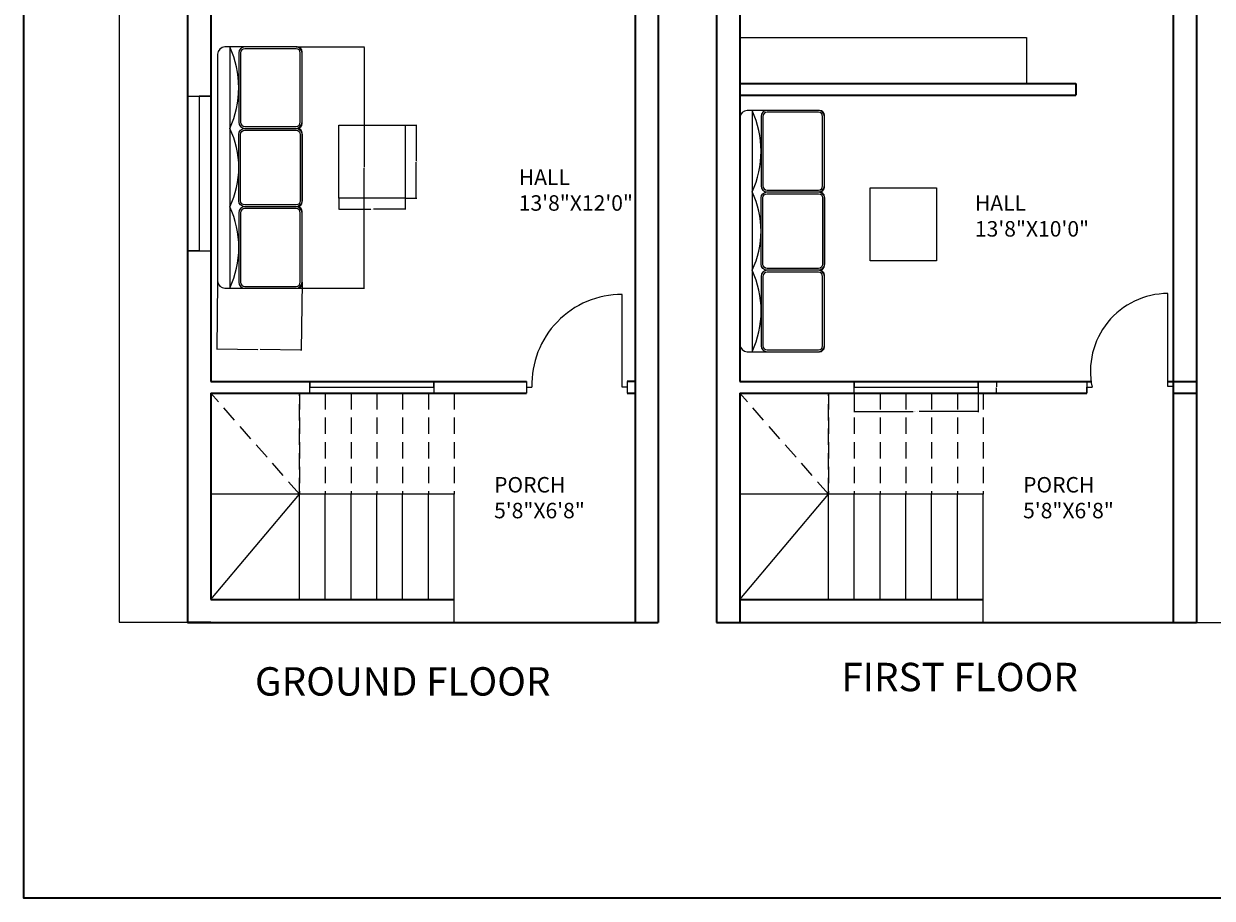
# Model space of a CAD drawing. Units: inches. Extents: x 2169 to 3181, y 1824 to 2912.
# Tile 1 of 5: x 2169 to 2630, y 1824 to 2163. Entities that reach past the tile are written whole.
import ezdxf

# ---------------------------------------------------------------- set-up
doc = ezdxf.new("R2010")
doc.units = ezdxf.units.IN
doc.linetypes.add('DASHED2', pattern=[9.525, 6.35, -3.175])
for name, color, linetype, lineweight in [('A-ANNO-DIMS', 2, 'Continuous', 18), ('A-ANNO-TITL', 7, 'Continuous', 25), ('A-ANNO-TTLB', 7, 'Continuous', 35), ('A-AREA-IDEN', 7, 'Continuous', 18), ('A-DOOR', 3, 'Continuous', 18), ('A-FLOR-CASE', 8, 'Continuous', 18), ('A-FLOR-STRS', 7, 'Continuous', 18), ('A-FLOR-STRS-OVHD', 253, 'DASHED2', 13), ('A-FURN', 8, 'Continuous', 18), ('A-GLAZ', 4, 'Continuous', 18), ('A-WALL', 7, 'Continuous', 35)]:
    doc.layers.add(name, color=color, linetype=linetype, lineweight=lineweight)
doc.styles.get("Standard").update_dxf_attribs({"font": 'arial.ttf'})
doc.dimstyles.get("Standard").update_dxf_attribs({"dimtxt": 0.18, "dimasz": 0.18, "dimexe": 0.18, "dimexo": 0.0625, "dimgap": 0.09, "dimtad": 0, "dimtih": 1, "dimtoh": 1, "dimdec": 4, "dimzin": 0, "dimdsep": 46, "dimtxsty": 'Standard', "dimcen": 0.09, "dimadec": 0, "dimazin": 0, "dimtfac": 1, "dimtdec": 4, "dimtofl": 0, "dimtmove": 0, "dimatfit": 3, "dimfxl": 1, "dimtolj": 1, "dimtzin": 0, "dimarcsym": 0})

# ---------------------------------------------------------------- blocks, each defined once
blk = doc.blocks.new('DOOR-ENTRY-G-36IN')
for p, q in [((0, 0), (0, 36)), ((-37.01, 2.25), (-37.01, -2.25)), ((2, 2.25), (2, -2.25)), ((-37.01, 0), (-35.01, 0)), ((2, 0), (0, 0))]:
    blk.add_line(p, q)
blk.add_arc((0, 0.98), 35.02, 90, 181.6016)
blk = doc.blocks.new('DOOR-ENTRY-U-36IN')
for p, q in [((0, 0), (0, 36)), ((-31.41, 1.93), (-31.41, 1.93)), ((-31.41, 1.93), (-31.41, -2.57)), ((2, 0), (0, 0)), ((-31.41, -2.57), (-31.41, -0.32)), ((-31.41, -0.32), (-31.41, -0.32)), ((-31.41, -0.32), (-29.41, -0.32))]:
    blk.add_line(p, q)
blk.add_arc((0, 5.93), 30.07, 90, 192.0072)
blk = doc.blocks.new('WIN-60IN')
for p, q in [((4.5, 60), (0, 60)), ((0, 60), (9, 60)), ((4.5, 0), (4.5, 60)), ((0, 0), (9, 0)), ((9, 0), (4.5, 0)), ((9, 0), (9, 0))]:
    blk.add_line(p, q)
blk = doc.blocks.new('WIN-48IN')
for p, q in [((0, 0), (0, 4.5)), ((0, 4.5), (0, 2.25)), ((0, 2.25), (48, 2.25)), ((48, 2.25), (48, 4.5)), ((48, 4.5), (48, 0))]:
    blk.add_line(p, q)
blk = doc.blocks.new('STAIR-RETURN-LOWER')
for p, q in [((94.36, 49.81), (0, 49.81)), ((0, 9), (34.36, 49.81)), ((34.36, 9), (34.36, 49.81)), ((44.36, 9), (44.36, 49.81)), ((54.36, 9), (54.36, 49.81)), ((64.36, 9), (64.36, 49.81)), ((74.36, 9), (74.36, 49.81)), ((84.36, 9), (84.36, 49.81)), ((94.36, 0), (94.36, 49.81))]:
    blk.add_line(p, q)
blk = doc.blocks.new('STAIR-RETURN-UPPER')
for p, q in [((34.36, 0), (0, 39.19)), ((34.36, 0), (34.36, 39.19)), ((34.36, 39.19), (34.36, 0)), ((44.36, 39.19), (44.36, 0)), ((54.36, 39.19), (54.36, 0)), ((64.36, 39.19), (64.36, 0)), ((74.36, 39.19), (74.36, 0)), ((84.36, 39.19), (84.36, 0)), ((94.36, 39.19), (94.36, 0))]:
    blk.add_line(p, q)
blk = doc.blocks.new('TABLE-COFFEE')
blk.add_lwpolyline([(0, 28.27), (25.7, 28.27), (25.7, 0), (0, 0)], close=True)
blk = doc.blocks.new('*D21')
at = {"layer": 'A-ANNO-DIMS', "color": 0, "lineweight": -2, "transparency": 16777216}
for p, q in [((2490.73, 2019.33), (2490.73, 2012.01)), ((2538.73, 2019.33), (2538.73, 2012.01)), ((2490.91, 2012.19), (2513.61, 2012.19)), ((2538.55, 2012.19), (2515.85, 2012.19))]:
    blk.add_line(p, q, dxfattribs=at)
at = {"layer": 'A-ANNO-DIMS', "color": 0, "transparency": 16777216}
for points in [[(2490.91, 2012.22), (2490.91, 2012.16), (2490.73, 2012.19)], [(2538.55, 2012.22), (2538.55, 2012.16), (2538.73, 2012.19)]]:
    blk.add_solid(points, dxfattribs=at)
at = {"layer": 'Defpoints', "color": 0, "transparency": 16777216}
for p in [(2490.73, 2019.39), (2538.73, 2019.39), (2538.73, 2012.19)]:
    blk.add_point(p, dxfattribs=at)
at = {"layer": 'A-ANNO-DIMS', "color": 0, "transparency": 16777216, "insert": (2514.73, 2012.19), "char_height": 0.18, "attachment_point": 5}
blk.add_mtext('\\A1;WINDOW 48 TYP.', dxfattribs=at)
blk = doc.blocks.new('*D22')
at = {"layer": 'A-ANNO-DIMS', "color": 0, "lineweight": -2, "transparency": 16777216}
for p, q in [((2538.8, 2023.89), (2546.11, 2023.89)), ((2545.93, 2023.71), (2545.93, 2021.82)), ((2538.8, 2019.39), (2546.11, 2019.39)), ((2545.93, 2019.57), (2545.93, 2021.46))]:
    blk.add_line(p, q, dxfattribs=at)
at = {"layer": 'A-ANNO-DIMS', "color": 0, "transparency": 16777216}
for points in [[(2545.9, 2023.71), (2545.96, 2023.71), (2545.93, 2023.89)], [(2545.9, 2019.57), (2545.96, 2019.57), (2545.93, 2019.39)]]:
    blk.add_solid(points, dxfattribs=at)
at = {"layer": 'Defpoints', "color": 0, "transparency": 16777216}
for p in [(2538.73, 2023.89), (2545.93, 2023.89), (2538.73, 2019.39)]:
    blk.add_point(p, dxfattribs=at)
at = {"layer": 'A-ANNO-DIMS', "color": 0, "transparency": 16777216, "insert": (2545.93, 2021.64), "char_height": 0.18, "attachment_point": 5}
blk.add_mtext('\\A1;5 TYP.', dxfattribs=at)
blk = doc.blocks.new('*D47')
at = {"layer": 'A-ANNO-DIMS', "color": 0, "lineweight": -2, "transparency": 16777216}
for p, q in [((2316.73, 2123.18), (2321.09, 2123.18)), ((2320.91, 2123), (2320.91, 2109.23)), ((2320.91, 2095.09), (2320.91, 2108.86)), ((2316.73, 2094.91), (2321.09, 2094.91))]:
    blk.add_line(p, q, dxfattribs=at)
at = {"layer": 'A-ANNO-DIMS', "color": 0, "transparency": 16777216}
for points in [[(2320.88, 2123), (2320.94, 2123), (2320.91, 2123.18)], [(2320.88, 2095.09), (2320.94, 2095.09), (2320.91, 2094.91)]]:
    blk.add_solid(points, dxfattribs=at)
at = {"layer": 'Defpoints', "color": 0, "transparency": 16777216}
for p in [(2316.67, 2123.18), (2320.91, 2123.18), (2316.67, 2094.91)]:
    blk.add_point(p, dxfattribs=at)
at = {"layer": 'A-ANNO-DIMS', "color": 0, "transparency": 16777216, "insert": (2320.91, 2109.04), "char_height": 0.18, "attachment_point": 5}
blk.add_mtext('\\A1;TABLE 28 TYP.', dxfattribs=at)
blk = doc.blocks.new('*D48')
at = {"layer": 'A-ANNO-DIMS', "color": 0, "lineweight": -2, "transparency": 16777216}
for p, q in [((2290.97, 2094.85), (2290.97, 2090.49)), ((2316.67, 2094.85), (2316.67, 2090.49)), ((2291.15, 2090.67), (2303.29, 2090.67)), ((2316.49, 2090.67), (2304.35, 2090.67))]:
    blk.add_line(p, q, dxfattribs=at)
at = {"layer": 'A-ANNO-DIMS', "color": 0, "transparency": 16777216}
for points in [[(2291.15, 2090.7), (2291.15, 2090.64), (2290.97, 2090.67)], [(2316.49, 2090.7), (2316.49, 2090.64), (2316.67, 2090.67)]]:
    blk.add_solid(points, dxfattribs=at)
at = {"layer": 'Defpoints', "color": 0, "transparency": 16777216}
for p in [(2290.97, 2094.91), (2316.67, 2094.91), (2316.67, 2090.67)]:
    blk.add_point(p, dxfattribs=at)
at = {"layer": 'A-ANNO-DIMS', "color": 0, "transparency": 16777216, "insert": (2303.82, 2090.67), "char_height": 0.18, "attachment_point": 5}
blk.add_mtext('\\A1;26 TYP.', dxfattribs=at)
blk = doc.blocks.new('*D54')
at = {"layer": 'A-ANNO-DIMS', "color": 0, "lineweight": -2, "transparency": 16777216}
for p, q in [((2232.21, 2417.39), (2205.74, 2417.39)), ((2205.92, 2417.21), (2205.92, 2174.07)), ((2205.92, 1930.57), (2205.92, 2173.71)), ((2232.21, 1930.39), (2205.74, 1930.39))]:
    blk.add_line(p, q, dxfattribs=at)
at = {"layer": 'A-ANNO-DIMS', "color": 0, "transparency": 16777216}
for points in [[(2205.89, 2417.21), (2205.95, 2417.21), (2205.92, 2417.39)], [(2205.89, 1930.57), (2205.95, 1930.57), (2205.92, 1930.39)]]:
    blk.add_solid(points, dxfattribs=at)
at = {"layer": 'Defpoints', "color": 0, "transparency": 16777216}
for p in [(2205.92, 2417.39), (2232.27, 2417.39), (2232.27, 1930.39)]:
    blk.add_point(p, dxfattribs=at)
at = {"layer": 'A-ANNO-DIMS', "color": 0, "transparency": 16777216, "insert": (2205.92, 2173.89), "char_height": 0.18, "attachment_point": 5}
blk.add_mtext('\\A1;487', dxfattribs=at)
blk = doc.blocks.new('*D56')
at = {"layer": 'A-ANNO-DIMS', "color": 0, "lineweight": -2, "transparency": 16777216}
for p, q in [((2623.43, 2417.39), (2649.9, 2417.39)), ((2649.72, 2417.21), (2649.72, 2174.07)), ((2649.72, 1930.57), (2649.72, 2173.71)), ((2623.43, 1930.39), (2649.9, 1930.39))]:
    blk.add_line(p, q, dxfattribs=at)
at = {"layer": 'A-ANNO-DIMS', "color": 0, "transparency": 16777216}
for points in [[(2649.69, 2417.21), (2649.75, 2417.21), (2649.72, 2417.39)], [(2649.69, 1930.57), (2649.75, 1930.57), (2649.72, 1930.39)]]:
    blk.add_solid(points, dxfattribs=at)
at = {"layer": 'Defpoints', "color": 0, "transparency": 16777216}
for p in [(2623.37, 2417.39), (2649.72, 2417.39), (2623.37, 1930.39)]:
    blk.add_point(p, dxfattribs=at)
at = {"layer": 'A-ANNO-DIMS', "color": 0, "transparency": 16777216, "insert": (2649.72, 2173.89), "char_height": 0.18, "attachment_point": 5}
blk.add_mtext('\\A1;487', dxfattribs=at)
blk = doc.blocks.new('*D62')
at = {"layer": 'A-ANNO-DIMS', "color": 0, "lineweight": -2, "transparency": 16777216}
for p, q in [((2243.93, 2062.78), (2243.55, 2036.32)), ((2276.66, 2062.31), (2276.28, 2035.85)), ((2243.73, 2036.5), (2259.46, 2036.27)), ((2276.1, 2036.03), (2260.38, 2036.26))]:
    blk.add_line(p, q, dxfattribs=at)
at = {"layer": 'A-ANNO-DIMS', "color": 0, "transparency": 16777216}
for points in [[(2243.74, 2036.53), (2243.73, 2036.47), (2243.55, 2036.5)], [(2276.11, 2036.06), (2276.1, 2036), (2276.28, 2036.03)]]:
    blk.add_solid(points, dxfattribs=at)
at = {"layer": 'Defpoints', "color": 0, "transparency": 16777216}
for p in [(2243.93, 2062.85), (2276.66, 2062.38), (2243.55, 2036.5)]:
    blk.add_point(p, dxfattribs=at)
at = {"layer": 'A-ANNO-DIMS', "color": 0, "transparency": 16777216, "insert": (2259.92, 2036.26), "char_height": 0.18, "attachment_point": 5}
blk.add_mtext('\\A1;32.733', dxfattribs=at)
blk = doc.blocks.new('*D63')
at = {"layer": 'A-ANNO-DIMS', "color": 0, "lineweight": -2, "transparency": 16777216}
for p, q in [((2274.39, 2153.55), (2300.85, 2153.55)), ((2300.67, 2153.37), (2300.67, 2106.98)), ((2300.67, 2060.22), (2300.67, 2106.61)), ((2274.39, 2060.04), (2300.85, 2060.04))]:
    blk.add_line(p, q, dxfattribs=at)
at = {"layer": 'A-ANNO-DIMS', "color": 0, "transparency": 16777216}
for points in [[(2300.64, 2153.37), (2300.7, 2153.37), (2300.67, 2153.55)], [(2300.64, 2060.22), (2300.7, 2060.22), (2300.67, 2060.04)]]:
    blk.add_solid(points, dxfattribs=at)
at = {"layer": 'Defpoints', "color": 0, "transparency": 16777216}
for p in [(2274.32, 2153.55), (2274.32, 2060.04), (2300.67, 2060.04)]:
    blk.add_point(p, dxfattribs=at)
at = {"layer": 'A-ANNO-DIMS', "color": 0, "transparency": 16777216, "insert": (2300.67, 2106.8), "char_height": 0.18, "attachment_point": 5}
blk.add_mtext('\\A1;93.51', dxfattribs=at)

msp = doc.modelspace()

# ---------------------------------------------------------------- linework, layer by layer
at = {"layer": 'A-ANNO-TTLB'}
msp.add_lwpolyline([(2168.7598, 2912.462), (3180.8253, 2912.462), (3180.8253, 1823.5481), (2168.7598, 1823.5481)], close=True, dxfattribs=at)
at = {"layer": 'A-FLOR-CASE'}
for p, q in [((2446.3698, 2157.1645), (2557.46, 2157.1645)), ((2557.46, 2157.1645), (2557.46, 2139.3924))]:
    msp.add_line(p, q, dxfattribs=at)
at = {"layer": 'A-FLOR-STRS'}
msp.add_line((2241.2736, 1939.3924), (2241.2736, 1939.3924), dxfattribs=at)
at = {"layer": 'A-FURN', "ltscale": 0.03}
for points in [[(2276.6613, 2123.8863), (2276.6613, 2151.6838, 0.41421356), (2274.791, 2153.5541), (2246.7367, 2153.5541, 0.41421356), (2243.9312, 2150.7487), (2243.9312, 2062.845, 0.41421356), (2246.7367, 2060.0396), (2274.791, 2060.0396, 0.41421356), (2276.6613, 2061.9099), (2276.6613, 2089.7075, 0.41421356), (2274.791, 2091.5778, -1), (2274.791, 2091.6237, 0.41421356), (2276.6613, 2093.494), (2276.6613, 2120.0997, 0.41421356), (2274.791, 2121.97, -1), (2274.791, 2122.016, 0.41421356)], [(2479.1674, 2099.2454), (2479.1674, 2127.043, 0.41421356), (2477.2971, 2128.9133), (2449.2428, 2128.9133, 0.41421356), (2446.4373, 2126.1078), (2446.4373, 2038.2042, 0.41421356), (2449.2428, 2035.3988), (2477.2971, 2035.3988, 0.41421356), (2479.1674, 2037.269), (2479.1674, 2065.0666, 0.41421356), (2477.2971, 2066.9369, -1), (2477.2971, 2066.9829, 0.41421356), (2479.1674, 2068.8532), (2479.1674, 2095.4588, 0.41421356), (2477.2971, 2097.3291, -1), (2477.2971, 2097.3751, 0.41421356)]]:
    msp.add_lwpolyline(points, format="xyb", close=True, dxfattribs=at)
at = {"layer": 'A-FURN'}
for points in [[(2248.607, 2153.5541), (2248.607, 2060.0396)], [(2451.1131, 2128.9133), (2451.1131, 2035.3988)]]:
    msp.add_lwpolyline(points, dxfattribs=at)
for points in [[(2274.3235, 2153.5541), (2254.4516, 2153.5541, 0.41421356), (2252.1138, 2151.2163), (2252.1138, 2124.3308, 0.41421356), (2254.4516, 2121.993), (2274.3235, 2121.993, 0.41421356), (2276.6613, 2124.3308), (2276.6613, 2151.2163, 0.41421356)], [(2274.3235, 2152.8528), (2254.4516, 2152.8528, 0.41421356), (2252.8151, 2151.2163), (2252.8151, 2124.3308, 0.41421356), (2254.4516, 2122.6943), (2274.3235, 2122.6943, 0.41421356), (2275.96, 2124.3308), (2275.96, 2151.2163, 0.41421356)], [(2476.8296, 2128.9133), (2456.9577, 2128.9133, 0.41421356), (2454.6199, 2126.5754), (2454.6199, 2099.69, 0.41421356), (2456.9577, 2097.3521), (2476.8296, 2097.3521, 0.41421356), (2479.1674, 2099.69), (2479.1674, 2126.5754, 0.41421356)], [(2476.8296, 2128.2119), (2456.9577, 2128.2119, 0.41421356), (2455.3212, 2126.5754), (2455.3212, 2099.69, 0.41421356), (2456.9577, 2098.0535), (2476.8296, 2098.0535, 0.41421356), (2478.4661, 2099.69), (2478.4661, 2126.5754, 0.41421356)], [(2274.3235, 2091.6008), (2254.4516, 2091.6008, -0.41421356), (2252.1138, 2093.9386), (2252.1138, 2119.6551, -0.41421356), (2254.4516, 2121.993), (2274.3235, 2121.993, -0.41421356), (2276.6613, 2119.6551), (2276.6613, 2093.9386, -0.41421356)], [(2274.3235, 2092.3021), (2254.4516, 2092.3021, -0.41421356), (2252.8151, 2093.9386), (2252.8151, 2119.6551, -0.41421356), (2254.4516, 2121.2916), (2274.3235, 2121.2916, -0.41421356), (2275.96, 2119.6551), (2275.96, 2093.9386, -0.41421356)], [(2476.8296, 2066.9599), (2456.9577, 2066.9599, -0.41421356), (2454.6199, 2069.2978), (2454.6199, 2095.0143, -0.41421356), (2456.9577, 2097.3521), (2476.8296, 2097.3521, -0.41421356), (2479.1674, 2095.0143), (2479.1674, 2069.2978, -0.41421356)], [(2476.8296, 2067.6613), (2456.9577, 2067.6613, -0.41421356), (2455.3212, 2069.2978), (2455.3212, 2095.0143, -0.41421356), (2456.9577, 2096.6508), (2476.8296, 2096.6508, -0.41421356), (2478.4661, 2095.0143), (2478.4661, 2069.2978, -0.41421356)], [(2274.3235, 2091.6008), (2254.4516, 2091.6008, 0.41421356), (2252.1138, 2089.2629), (2252.1138, 2062.3775, 0.41421356), (2254.4516, 2060.0396), (2274.3235, 2060.0396, 0.41421356), (2276.6613, 2062.3775), (2276.6613, 2089.2629, 0.41421356)], [(2274.3235, 2090.8994), (2254.4516, 2090.8994, 0.41421356), (2252.8151, 2089.2629), (2252.8151, 2062.3775, 0.41421356), (2254.4516, 2060.741), (2274.3235, 2060.741, 0.41421356), (2275.96, 2062.3775), (2275.96, 2089.2629, 0.41421356)], [(2476.8296, 2066.9599), (2456.9577, 2066.9599, 0.41421356), (2454.6199, 2064.622), (2454.6199, 2037.7366, 0.41421356), (2456.9577, 2035.3988), (2476.8296, 2035.3988, 0.41421356), (2479.1674, 2037.7366), (2479.1674, 2064.622, 0.41421356)], [(2476.8296, 2066.2585), (2456.9577, 2066.2585, 0.41421356), (2455.3212, 2064.622), (2455.3212, 2037.7366, 0.41421356), (2456.9577, 2036.1001), (2476.8296, 2036.1001, 0.41421356), (2478.4661, 2037.7366), (2478.4661, 2064.622, 0.41421356)]]:
    msp.add_lwpolyline(points, format="xyb", close=True, dxfattribs=at)
for centre, radius, start, end in [((2214.9028, 2137.7736), 37.2156, 334.910626, 25.089374), ((2417.4089, 2113.1327), 37.2156, 334.910626, 25.089374), ((2217.6303, 2106.7969), 34.5033, 333.868999, 26.131001), ((2420.1364, 2082.156), 34.5033, 333.868999, 26.131001), ((2215.2924, 2075.8202), 36.8631, 334.653824, 25.346176), ((2417.7985, 2051.1793), 36.8631, 334.653824, 25.346176)]:
    msp.add_arc(centre, radius, start, end, dxfattribs=at)
at = {"layer": 'A-GLAZ'}
msp.add_line((2490.7332, 2019.3924), (2490.7332, 2019.3924), dxfattribs=at)
at = {"layer": 'A-WALL'}
for p, q in [((2232.2736, 2417.3924), (2232.2736, 1930.3924)), ((2414.7736, 2417.3924), (2414.7736, 1930.3924)), ((2437.3698, 2417.3924), (2437.3698, 1930.3924)), ((2623.3698, 2417.3924), (2623.3698, 1930.3924)), ((2446.3698, 2408.3924), (2446.3698, 2023.8924)), ((2614.3698, 2408.3924), (2614.3698, 1930.3924)), ((2241.2736, 2319.8924), (2241.2736, 2023.8924)), ((2405.7736, 2263.8924), (2405.7736, 1930.3924)), ((2446.3698, 2139.3924), (2576.6687, 2139.3924)), ((2576.6687, 2139.3924), (2576.6687, 2139.3924)), ((2576.6687, 2139.3924), (2576.6687, 2134.8924)), ((2446.3698, 2134.8924), (2576.6687, 2134.8924)), ((2241.2736, 2023.8924), (2363.7249, 2023.8924)), ((2405.7736, 2023.8924), (2402.7324, 2023.8924)), ((2446.3698, 2023.8924), (2582.5713, 2023.8924)), ((2612.3698, 2023.8924), (2623.3698, 2023.8924)), ((2241.2736, 2019.3924), (2363.7249, 2019.3924)), ((2241.2736, 2019.3924), (2241.2736, 1939.3924)), ((2402.7324, 2019.3924), (2405.7736, 2019.3924)), ((2446.3698, 2019.3924), (2580.9612, 2019.3924)), ((2446.3698, 2019.3924), (2446.3698, 1930.3924)), ((2614.3698, 2019.3924), (2623.3698, 2019.3924)), ((2241.2736, 1939.3924), (2335.637, 1939.3924)), ((2446.3698, 1939.3924), (2540.7332, 1939.3924)), ((2241.2736, 1930.3924), (2232.2736, 1930.3924)), ((2232.2736, 1930.3924), (2414.7736, 1930.3924)), ((2241.2736, 1930.3924), (2335.637, 1930.3924)), ((2437.3698, 1930.3924), (2623.3698, 1930.3924)), ((2623.3698, 1930.3924), (2623.3698, 1930.3924))]:
    msp.add_line(p, q, dxfattribs=at)

# ---------------------------------------------------------------- block references
at = {"layer": 'A-DOOR'}
for name, p in [('DOOR-ENTRY-G-36IN', (2400.7324, 2021.6424)), ('DOOR-ENTRY-U-36IN', (2612.3698, 2021.9638))]:
    msp.add_blockref(name, p, dxfattribs=at)
at = {"layer": 'A-FLOR-STRS'}
for p in [(2241.274, 1930.392), (2446.3702, 1930.392), (2446.3702, 1930.392)]:
    msp.add_blockref('STAIR-RETURN-LOWER', p, dxfattribs=at)
at = {"layer": 'A-FLOR-STRS-OVHD'}
for p in [(2241.274, 1980.202), (2446.3702, 1980.202), (2446.3702, 1980.202)]:
    msp.add_blockref('STAIR-RETURN-UPPER', p, dxfattribs=at)
at = {"layer": 'A-FURN'}
for p in [(2290.967, 2094.908), (2496.8831, 2070.6236)]:
    msp.add_blockref('TABLE-COFFEE', p, dxfattribs=at)
at = {"layer": 'A-GLAZ', "extrusion": (0, 0, -1), "zscale": -1, "rotation": 180}
msp.add_blockref('WIN-60IN', (-2232.274, 2134.5134), dxfattribs=at)
at = {"layer": 'A-GLAZ'}
for p in [(2279.699, 2019.392), (2490.733, 2019.392)]:
    msp.add_blockref('WIN-48IN', p, dxfattribs=at)

# ---------------------------------------------------------------- texts
at = {"layer": 'A-ANNO-TITL', "char_height": 11, "attachment_point": 1}
for s, width, insert in [('GROUND FLOOR ', 160.442923, (2258.3886, 1913.1057)), ('FIRST FLOOR', 247.657349, (2485.7042, 1914.8003))]:
    msp.add_mtext_dynamic_manual_height_columns(s, width=width, gutter_width=12.5, heights=[0], dxfattribs=dict(at, insert=insert))
at = {"layer": 'A-AREA-IDEN', "char_height": 6, "attachment_point": 1}
for s, width, insert in [('HALL\\P13\'8"X12\'0"', 200.515112, (2360.6734, 2106.0569)), ('HALL\\P13\'8"X10\'0"', 142.922903, (2537.5221, 2096.0314)), ('PORCH\\P5\'8"X6\'8"', 130.589105, (2351.1073, 1986.8272)), ('PORCH\\P5\'8"X6\'8"', 130.589105, (2556.2035, 1986.8272)), ('PORCH\\P5\'8"X6\'8"', 130.589105, (2556.2035, 1986.8272))]:
    msp.add_mtext_dynamic_manual_height_columns(s, width=width, gutter_width=12.5, heights=[0], dxfattribs=dict(at, insert=insert))

# ---------------------------------------------------------------- dimensions: what is measured, and where the dimension line sits
at = {"layer": 'A-ANNO-DIMS'}
for base, p1, p2, angle, override, picture, middle in [((2205.9236, 2417.3924), (2232.2736, 1930.3924), (2232.2736, 2417.3924), 90, {"dimdec": 0, "dimlfac": 1, "dimrnd": 0, "dimzin": 0, "dimdsep": 46, "dimlunit": 2}, '*D54', (2205.9236, 2173.8924)), ((2649.7198, 2417.3924), (2623.3698, 1930.3924), (2623.3698, 2417.3924), 90, {"dimdec": 0, "dimlfac": 1, "dimrnd": 0, "dimzin": 0, "dimdsep": 46, "dimlunit": 2}, '*D56', (2649.7198, 2173.8924)), ((2300.6735, 2060.0396), (2274.3235, 2153.5541), (2274.3235, 2060.0396), 270, {"dimdec": 2, "dimlfac": 1, "dimrnd": 0, "dimzin": 0, "dimdsep": 46, "dimlunit": 2}, '*D63', (2300.6735, 2106.7969)), ((2243.5549, 2036.4977), (2276.6613, 2062.3775), (2243.9312, 2062.845), 179.181545, {"dimdec": 3, "dimlfac": 1, "dimrnd": 0, "dimzin": 0, "dimdsep": 46, "dimlunit": 2}, '*D62', (2259.9199, 2036.2639))]:
    dim = msp.add_linear_dim(base=base, p1=p1, p2=p2, angle=angle, dimstyle='Standard', override=override, dxfattribs=at)
    dim.commit()
    dim.dimension.update_dxf_attribs({"geometry": picture, "text_midpoint": middle})
for base, p1, p2, text, picture, middle in [((2320.9085, 2123.1803), (2316.6676, 2094.9077), (2316.6676, 2123.1803), 'TABLE <> TYP.', '*D47', (2320.9085, 2109.044)), ((2545.9331818425, 2023.8923951293), (2538.7331818425, 2019.3923951293), (2538.7331818425, 2023.8923951293), '<> TYP.', '*D22', (2545.9331818425, 2021.6423951293))]:
    dim = msp.add_linear_dim(base=base, p1=p1, p2=p2, angle=90, text=text, dimstyle='Standard', override={"dimdec": 0, "dimlfac": 1, "dimrnd": 0, "dimzin": 0, "dimdsep": 46, "dimlunit": 2}, dxfattribs=at)
    dim.commit()
    dim.dimension.update_dxf_attribs({"geometry": picture, "text_midpoint": middle})
for base, p1, p2, text, picture, middle in [((2316.6676, 2090.6668), (2290.9669, 2094.9077), (2316.6676, 2094.9077), '<> TYP.', '*D48', (2303.8172, 2090.6668)), ((2538.7332, 2012.1924), (2490.7332, 2019.3924), (2538.7332, 2019.3924), 'WINDOW <> TYP.', '*D21', (2514.7332, 2012.1924))]:
    dim = msp.add_linear_dim(base=base, p1=p1, p2=p2, text=text, dimstyle='Standard', override={"dimdec": 0, "dimlfac": 1, "dimrnd": 0, "dimzin": 0, "dimdsep": 46, "dimlunit": 2}, dxfattribs=at)
    dim.commit()
    dim.dimension.update_dxf_attribs({"geometry": picture, "text_midpoint": middle})

doc.saveas('drawing.dxf')
